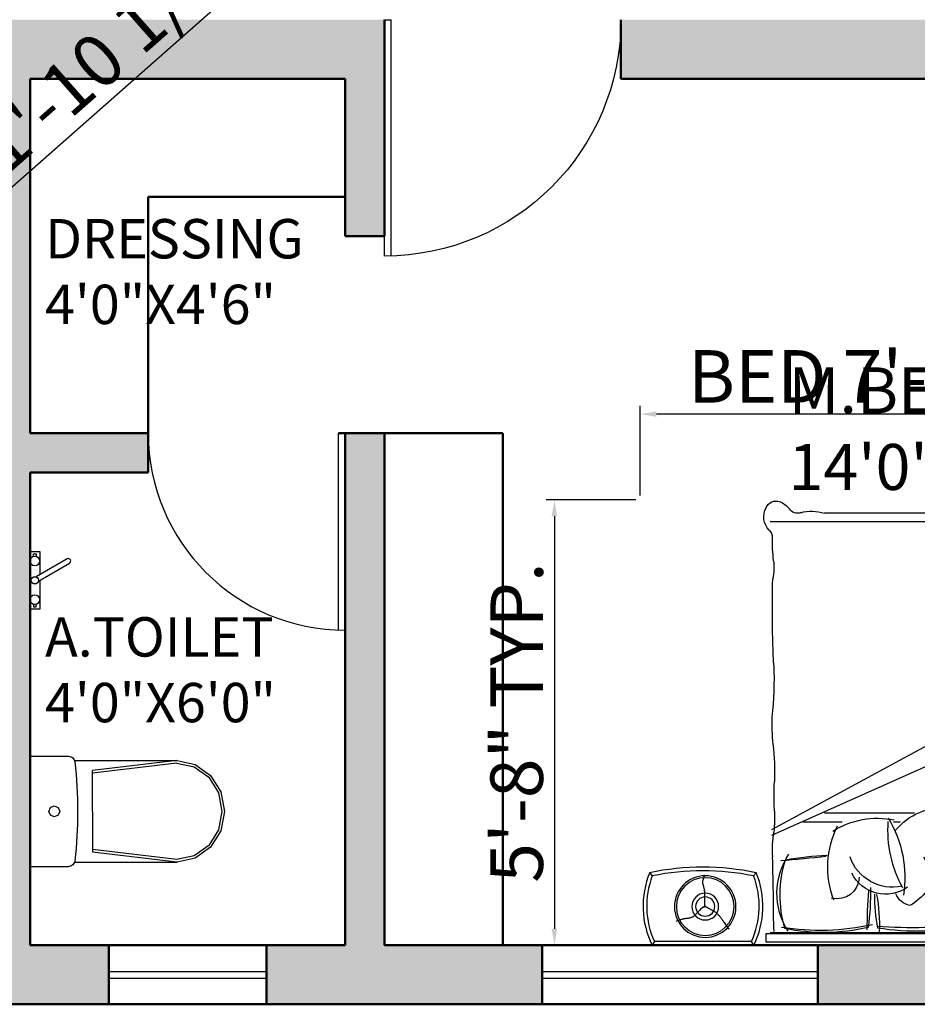
# Model space of a CAD drawing. Units: inches. Extents: x 3008 to 4088, y 1255 to 2137.
# Tile 23 of 30: x 3796 to 3933, y 1470 to 1620. Entities that reach past the tile are written whole.
import ezdxf

# ---------------------------------------------------------------- set-up
doc = ezdxf.new("R2010")
doc.units = ezdxf.units.IN
for name, color, linetype, lineweight in [('A-ANNO-DIMS', 2, 'Continuous', 18), ('A-AREA-IDEN', 7, 'Continuous', 18), ('A-DOOR', 4, 'Continuous', 25), ('A-FLOR-FIXT', 8, 'Continuous', 18), ('A-FURN', 8, 'Continuous', 18), ('A-GLAZ', 4, 'Continuous', 25), ('A-WALL', 7, 'Continuous', 50), ('A-WALL-PATT', 8, 'Continuous', 13)]:
    doc.layers.add(name, color=color, linetype=linetype, lineweight=lineweight)
doc.layers.add('SANTEH', color=7, linetype='Continuous')
doc.layers.add('TEFRİŞ', color=11, linetype='Continuous')
doc.styles.get("Standard").update_dxf_attribs({"font": 'arial.ttf'})
doc.dimstyles.new('ISO-25', dxfattribs={"dimtxt": 8, "dimasz": 2.5, "dimexe": 1.25, "dimexo": 0.625, "dimtad": 1, "dimdec": 1, "dimlunit": 3, "dimtxsty": 'Standard', "dimcen": 2.5, "dimadec": 0, "dimazin": 0, "dimtfac": 1, "dimtdec": 1, "dimtmove": 0, "dimatfit": 3, "dimfxl": 1, "dimarcsym": 0})

# ---------------------------------------------------------------- blocks, each defined once
blk = doc.blocks.new('D1')
for p, q in [((1805.96, 1500.36), (1805.96, 1464.36)), ((1806.96, 1500.36), (1806.96, 1464.36)), ((1805.96, 1464.36), (1806.96, 1464.36))]:
    blk.add_line(p, q)
blk.add_arc((1805.96, 1464.36), 36, 0, 90)
blk = doc.blocks.new('D2')
for p, q in [((1722.5, 1505.46), (1722.5, 1475.46)), ((1723.5, 1505.46), (1723.5, 1475.46)), ((1722.5, 1475.46), (1723.5, 1475.46))]:
    blk.add_line(p, q)
blk.add_arc((1722.5, 1475.46), 30, 0, 90)
blk = doc.blocks.new('WC 2 Symb_109')
at = {"layer": 'SANTEH'}
for p, q in [((0, 0), (0, 380)), ((0, 380), (132.4, 380)), ((153.6, 364.9), (506.8, 364.9)), ((506.3, 364.9), (215.7, 330.9)), ((506.3, 356), (215.7, 322)), ((215.7, 190), (215.7, 330.9)), ((215.7, 190), (215.7, 49.1)), ((506.3, 24), (215.7, 58)), ((506.3, 15.1), (215.7, 49.1)), ((153.8, 15.1), (506.8, 15.1)), ((0, 0), (132.4, 0))]:
    blk.add_line(p, q, dxfattribs=at)
for points in [[(154.6, 360.1), (153.9, 364.1), (152.3, 367.9), (150.2, 371.3), (147.4, 374.3), (144.1, 376.7), (140.5, 378.5), (136.5, 379.6), (132.4, 380)], [(154.6, 19.7), (158.6, 62.1), (161.4, 104.7), (163.1, 147.3), (163.7, 189.9), (163.1, 232.5), (161.4, 275.1), (158.6, 317.7), (154.6, 360.1)], [(506.3, 24), (565.5, 36.6), (615.7, 72.6), (649.2, 126.5), (661, 190), (649.2, 253.5), (615.7, 307.4), (565.5, 343.4), (506.3, 356)], [(506.8, 15.1), (569.2, 28.4), (622.2, 66.3), (657.6, 123.1), (670, 190), (657.6, 256.9), (622.2, 313.7), (569.2, 351.6), (506.8, 364.9)], [(132.4, 0), (136.5, 0.4), (140.4, 1.5), (144.1, 3.2), (147.3, 5.6), (150.1, 8.6), (152.3, 12), (153.8, 15.7), (154.6, 19.7)]]:
    blk.add_lwpolyline(points, dxfattribs=at)
blk.add_lwpolyline([(83.6, 208.5), (70.4, 203.1), (64.9, 190), (70.4, 176.9), (83.6, 171.5), (96.8, 176.9), (102.2, 190), (96.8, 203.1)], close=True, dxfattribs=at)
blk = doc.blocks.new('Faucet - kit sink top')
at = {"layer": 'SANTEH'}
for p, q in [((-5.5, -0.75), (-5.5, -1.25)), ((-4.94278, -0.75), (-5.5, -0.75)), ((-5.5, -1.25), (-4.94278, -1.25)), ((-0.14775, -1.7441), (3.56698, -8.1782)), ((4.43301, -7.6782), (0.71828, -1.2441)), ((4.94278, -0.75), (5.5, -0.75)), ((5.5, -1.25), (4.94278, -1.25)), ((5.5, -0.75), (5.5, -1.25))]:
    blk.add_line(p, q, dxfattribs=at)
blk.add_lwpolyline([(-0.00587, -2), (-6, -2), (-6, 0), (6, 0), (6, -2), (1.15195, -2)], dxfattribs=at)
for centre, radius in [((-4, -1), 1), ((4, -1), 1), ((0, -1), 0.75)]:
    blk.add_circle(centre, radius, dxfattribs=at)
blk.add_arc((4, -7.9282), 0.5, 210, 30, dxfattribs=at)
blk = doc.blocks.new('BED')
at = {"layer": 'TEFRİŞ'}
for p, q in [((2114.88, 1835.66), (2129.12, 1835.66)), ((2130.81, 1834.34), (2130.81, 1835.55)), ((2130.91, 1835.55), (2175.56, 1835.55)), ((2175.56, 1835.55), (2175.56, 1834.34)), ((2177.29, 1835.98), (2177.61, 1835.47)), ((2177.29, 1835.98), (2191.52, 1835.98)), ((2191.2, 1835.47), (2191.52, 1835.98)), ((2115.2, 1835.15), (2128.8, 1835.15)), ((2175.56, 1834.34), (2130.81, 1834.34)), ((2175, 1834.19), (2130.91, 1834.19)), ((2177.61, 1835.47), (2191.2, 1835.47)), ((2118.49, 1833.2), (2118.34, 1833.38)), ((2118.49, 1833.2), (2118.34, 1833.38)), ((2118.63, 1833.03), (2118.49, 1833.2)), ((2118.63, 1833.03), (2118.49, 1833.2)), ((2118.75, 1832.88), (2118.63, 1833.03)), ((2118.75, 1832.88), (2118.63, 1833.03)), ((2118.86, 1832.74), (2118.75, 1832.88)), ((2118.86, 1832.74), (2118.75, 1832.88)), ((2180.9, 1833.52), (2180.75, 1833.7)), ((2180.9, 1833.52), (2180.75, 1833.7)), ((2181.04, 1833.35), (2180.9, 1833.52)), ((2181.04, 1833.35), (2180.9, 1833.52)), ((2181.16, 1833.2), (2181.04, 1833.35)), ((2181.16, 1833.2), (2181.04, 1833.35)), ((2181.26, 1833.06), (2181.16, 1833.2)), ((2181.26, 1833.06), (2181.16, 1833.2)), ((2181.36, 1832.93), (2181.26, 1833.06)), ((2181.36, 1832.93), (2181.26, 1833.06)), ((2181.44, 1832.8), (2181.36, 1832.93)), ((2181.44, 1832.8), (2181.36, 1832.93)), ((2181.52, 1832.69), (2181.44, 1832.8)), ((2181.52, 1832.69), (2181.44, 1832.8)), ((2118.95, 1832.61), (2118.86, 1832.74)), ((2118.95, 1832.61), (2118.86, 1832.74)), ((2119.04, 1832.48), (2118.95, 1832.61)), ((2119.04, 1832.48), (2118.95, 1832.61)), ((2119.12, 1832.37), (2119.04, 1832.48)), ((2119.12, 1832.37), (2119.04, 1832.48)), ((2119.19, 1832.26), (2119.12, 1832.37)), ((2119.19, 1832.26), (2119.12, 1832.37)), ((2119.26, 1832.16), (2119.19, 1832.26)), ((2119.26, 1832.16), (2119.19, 1832.26)), ((2119.32, 1832.06), (2119.26, 1832.16)), ((2119.32, 1832.06), (2119.26, 1832.16)), ((2119.39, 1831.97), (2119.32, 1832.06)), ((2119.39, 1831.97), (2119.32, 1832.06)), ((2119.45, 1831.89), (2119.39, 1831.97)), ((2119.45, 1831.89), (2119.39, 1831.97)), ((2119.51, 1831.81), (2119.45, 1831.89)), ((2119.51, 1831.81), (2119.45, 1831.89)), ((2119.57, 1831.73), (2119.51, 1831.81)), ((2119.57, 1831.73), (2119.51, 1831.81)), ((2119.63, 1831.65), (2119.57, 1831.73)), ((2119.63, 1831.65), (2119.57, 1831.73)), ((2119.69, 1831.58), (2119.63, 1831.65)), ((2119.69, 1831.58), (2119.63, 1831.65)), ((2119.75, 1831.51), (2119.69, 1831.58)), ((2119.75, 1831.51), (2119.69, 1831.58)), ((2119.81, 1831.44), (2119.75, 1831.51)), ((2119.81, 1831.44), (2119.75, 1831.51)), ((2119.87, 1831.38), (2119.81, 1831.44)), ((2119.87, 1831.38), (2119.81, 1831.44)), ((2123.01, 1831.33), (2123.08, 1831.4)), ((2123.01, 1831.33), (2123.08, 1831.4)), ((2123.08, 1831.4), (2123.14, 1831.46)), ((2123.08, 1831.4), (2123.14, 1831.46)), ((2123.14, 1831.46), (2123.21, 1831.52)), ((2123.14, 1831.46), (2123.21, 1831.52)), ((2123.21, 1831.52), (2123.27, 1831.58)), ((2123.21, 1831.52), (2123.27, 1831.58)), ((2123.27, 1831.58), (2123.34, 1831.63)), ((2123.27, 1831.58), (2123.34, 1831.63)), ((2123.34, 1831.63), (2123.41, 1831.67)), ((2123.34, 1831.63), (2123.41, 1831.67)), ((2123.41, 1831.67), (2123.48, 1831.71)), ((2123.41, 1831.67), (2123.48, 1831.71)), ((2123.48, 1831.71), (2123.55, 1831.74)), ((2123.48, 1831.71), (2123.55, 1831.74)), ((2123.55, 1831.74), (2123.62, 1831.77)), ((2123.55, 1831.74), (2123.62, 1831.77)), ((2123.62, 1831.77), (2123.69, 1831.8)), ((2123.62, 1831.77), (2123.69, 1831.8)), ((2123.69, 1831.8), (2123.77, 1831.82)), ((2123.69, 1831.8), (2123.77, 1831.82)), ((2123.77, 1831.82), (2123.84, 1831.84)), ((2123.77, 1831.82), (2123.84, 1831.84)), ((2123.84, 1831.84), (2123.91, 1831.86)), ((2123.84, 1831.84), (2123.91, 1831.86)), ((2123.91, 1831.86), (2123.98, 1831.87)), ((2123.91, 1831.86), (2123.98, 1831.87)), ((2123.98, 1831.87), (2124.06, 1831.89)), ((2123.98, 1831.87), (2124.06, 1831.89)), ((2124.06, 1831.89), (2124.13, 1831.9)), ((2124.06, 1831.89), (2124.13, 1831.9)), ((2124.13, 1831.9), (2124.2, 1831.91)), ((2124.13, 1831.9), (2124.2, 1831.91)), ((2124.2, 1831.91), (2124.27, 1831.91)), ((2124.2, 1831.91), (2124.27, 1831.91)), ((2124.27, 1831.91), (2124.35, 1831.92)), ((2124.27, 1831.91), (2124.35, 1831.92)), ((2124.35, 1831.92), (2124.42, 1831.93)), ((2124.35, 1831.92), (2124.42, 1831.93)), ((2124.42, 1831.93), (2124.49, 1831.94)), ((2124.42, 1831.93), (2124.49, 1831.94)), ((2124.49, 1831.94), (2124.56, 1831.95)), ((2124.49, 1831.94), (2124.56, 1831.95)), ((2124.56, 1831.95), (2124.64, 1831.96)), ((2124.56, 1831.95), (2124.64, 1831.96)), ((2124.64, 1831.96), (2124.71, 1831.98)), ((2124.64, 1831.96), (2124.71, 1831.98)), ((2124.71, 1831.98), (2124.79, 1831.99)), ((2124.71, 1831.98), (2124.79, 1831.99)), ((2124.79, 1831.99), (2124.87, 1832.01)), ((2124.79, 1831.99), (2124.87, 1832.01)), ((2124.87, 1832.01), (2124.96, 1832.03)), ((2124.87, 1832.01), (2124.96, 1832.03)), ((2124.96, 1832.03), (2125.05, 1832.05)), ((2124.96, 1832.03), (2125.05, 1832.05)), ((2125.05, 1832.05), (2125.14, 1832.08)), ((2125.05, 1832.05), (2125.14, 1832.08)), ((2125.14, 1832.08), (2125.23, 1832.11)), ((2125.14, 1832.08), (2125.23, 1832.11)), ((2125.23, 1832.11), (2125.33, 1832.14)), ((2125.23, 1832.11), (2125.33, 1832.14)), ((2125.33, 1832.14), (2125.42, 1832.17)), ((2125.33, 1832.14), (2125.42, 1832.17)), ((2125.42, 1832.17), (2125.52, 1832.21)), ((2125.42, 1832.17), (2125.52, 1832.21)), ((2125.52, 1832.21), (2125.6, 1832.25)), ((2125.52, 1832.21), (2125.6, 1832.25)), ((2125.6, 1832.25), (2125.68, 1832.3)), ((2125.6, 1832.25), (2125.68, 1832.3)), ((2125.68, 1832.3), (2125.75, 1832.35)), ((2125.68, 1832.3), (2125.75, 1832.35)), ((2181.59, 1832.58), (2181.52, 1832.69)), ((2181.59, 1832.58), (2181.52, 1832.69)), ((2181.66, 1832.48), (2181.59, 1832.58)), ((2181.66, 1832.48), (2181.59, 1832.58)), ((2181.73, 1832.38), (2181.66, 1832.48)), ((2181.73, 1832.38), (2181.66, 1832.48)), ((2181.79, 1832.29), (2181.73, 1832.38)), ((2181.79, 1832.29), (2181.73, 1832.38)), ((2181.85, 1832.21), (2181.79, 1832.29)), ((2181.85, 1832.21), (2181.79, 1832.29)), ((2181.92, 1832.13), (2181.85, 1832.21)), ((2181.92, 1832.13), (2181.85, 1832.21)), ((2181.97, 1832.05), (2181.92, 1832.13)), ((2181.97, 1832.05), (2181.92, 1832.13)), ((2182.03, 1831.97), (2181.97, 1832.05)), ((2182.03, 1831.97), (2181.97, 1832.05)), ((2182.09, 1831.9), (2182.03, 1831.97)), ((2182.09, 1831.9), (2182.03, 1831.97)), ((2182.15, 1831.83), (2182.09, 1831.9)), ((2182.15, 1831.83), (2182.09, 1831.9)), ((2182.21, 1831.76), (2182.15, 1831.83)), ((2182.21, 1831.76), (2182.15, 1831.83)), ((2182.27, 1831.7), (2182.21, 1831.76)), ((2182.27, 1831.7), (2182.21, 1831.76)), ((2182.33, 1831.63), (2182.27, 1831.7)), ((2182.33, 1831.63), (2182.27, 1831.7)), ((2182.4, 1831.57), (2182.33, 1831.63)), ((2182.4, 1831.57), (2182.33, 1831.63)), ((2182.46, 1831.52), (2182.4, 1831.57)), ((2182.46, 1831.52), (2182.4, 1831.57)), ((2182.52, 1831.46), (2182.46, 1831.52)), ((2182.52, 1831.46), (2182.46, 1831.52)), ((2182.59, 1831.41), (2182.52, 1831.46)), ((2182.59, 1831.41), (2182.52, 1831.46)), ((2182.66, 1831.36), (2182.59, 1831.41)), ((2182.66, 1831.36), (2182.59, 1831.41)), ((2185.13, 1831.33), (2185.21, 1831.41)), ((2185.13, 1831.33), (2185.21, 1831.41)), ((2185.21, 1831.41), (2185.28, 1831.5)), ((2185.21, 1831.41), (2185.28, 1831.5)), ((2185.28, 1831.5), (2185.35, 1831.58)), ((2185.28, 1831.5), (2185.35, 1831.58)), ((2185.35, 1831.58), (2185.42, 1831.65)), ((2185.35, 1831.58), (2185.42, 1831.65)), ((2185.42, 1831.65), (2185.48, 1831.72)), ((2185.42, 1831.65), (2185.48, 1831.72)), ((2185.48, 1831.72), (2185.55, 1831.78)), ((2185.48, 1831.72), (2185.55, 1831.78)), ((2185.55, 1831.78), (2185.61, 1831.84)), ((2185.55, 1831.78), (2185.61, 1831.84)), ((2185.61, 1831.84), (2185.68, 1831.9)), ((2185.61, 1831.84), (2185.68, 1831.9)), ((2185.68, 1831.9), (2185.75, 1831.95)), ((2185.68, 1831.9), (2185.75, 1831.95)), ((2185.75, 1831.95), (2185.82, 1831.99)), ((2185.75, 1831.95), (2185.82, 1831.99)), ((2185.82, 1831.99), (2185.89, 1832.03)), ((2185.82, 1831.99), (2185.89, 1832.03)), ((2185.89, 1832.03), (2185.96, 1832.06)), ((2185.89, 1832.03), (2185.96, 1832.06)), ((2185.96, 1832.06), (2186.03, 1832.09)), ((2185.96, 1832.06), (2186.03, 1832.09)), ((2186.03, 1832.09), (2186.1, 1832.12)), ((2186.03, 1832.09), (2186.1, 1832.12)), ((2186.1, 1832.12), (2186.17, 1832.14)), ((2186.1, 1832.12), (2186.17, 1832.14)), ((2186.17, 1832.14), (2186.24, 1832.16)), ((2186.17, 1832.14), (2186.24, 1832.16)), ((2186.24, 1832.16), (2186.32, 1832.18)), ((2186.24, 1832.16), (2186.32, 1832.18)), ((2186.32, 1832.18), (2186.39, 1832.19)), ((2186.32, 1832.18), (2186.39, 1832.19)), ((2186.39, 1832.19), (2186.46, 1832.21)), ((2186.39, 1832.19), (2186.46, 1832.21)), ((2186.46, 1832.21), (2186.53, 1832.22)), ((2186.46, 1832.21), (2186.53, 1832.22)), ((2186.53, 1832.22), (2186.61, 1832.23)), ((2186.53, 1832.22), (2186.61, 1832.23)), ((2186.61, 1832.23), (2186.68, 1832.23)), ((2186.61, 1832.23), (2186.68, 1832.23)), ((2186.68, 1832.23), (2186.75, 1832.24)), ((2186.68, 1832.23), (2186.75, 1832.24)), ((2186.75, 1832.24), (2186.82, 1832.25)), ((2186.75, 1832.24), (2186.82, 1832.25)), ((2186.82, 1832.25), (2186.9, 1832.26)), ((2186.82, 1832.25), (2186.9, 1832.26)), ((2186.9, 1832.26), (2186.97, 1832.27)), ((2186.9, 1832.26), (2186.97, 1832.27)), ((2186.97, 1832.27), (2187.04, 1832.28)), ((2186.97, 1832.27), (2187.04, 1832.28)), ((2187.04, 1832.28), (2187.12, 1832.3)), ((2187.04, 1832.28), (2187.12, 1832.3)), ((2187.12, 1832.3), (2187.2, 1832.31)), ((2187.12, 1832.3), (2187.2, 1832.31)), ((2187.2, 1832.31), (2187.28, 1832.33)), ((2187.2, 1832.31), (2187.28, 1832.33)), ((2187.28, 1832.33), (2187.36, 1832.35)), ((2187.28, 1832.33), (2187.36, 1832.35)), ((2187.36, 1832.35), (2187.45, 1832.37)), ((2187.36, 1832.35), (2187.45, 1832.37)), ((2187.45, 1832.37), (2187.54, 1832.4)), ((2187.45, 1832.37), (2187.54, 1832.4)), ((2187.54, 1832.4), (2187.64, 1832.43)), ((2187.54, 1832.4), (2187.64, 1832.43)), ((2187.64, 1832.43), (2187.74, 1832.46)), ((2187.64, 1832.43), (2187.74, 1832.46)), ((2187.74, 1832.46), (2187.83, 1832.49)), ((2187.74, 1832.46), (2187.83, 1832.49)), ((2187.83, 1832.49), (2187.92, 1832.53)), ((2187.83, 1832.49), (2187.92, 1832.53)), ((2187.92, 1832.53), (2188.01, 1832.57)), ((2187.92, 1832.53), (2188.01, 1832.57)), ((2188.01, 1832.57), (2188.09, 1832.62)), ((2188.01, 1832.57), (2188.09, 1832.62)), ((2188.09, 1832.62), (2188.15, 1832.67)), ((2188.09, 1832.62), (2188.15, 1832.67)), ((2119.93, 1831.31), (2119.87, 1831.38)), ((2119.93, 1831.31), (2119.87, 1831.38)), ((2119.99, 1831.25), (2119.93, 1831.31)), ((2119.99, 1831.25), (2119.93, 1831.31)), ((2120.05, 1831.2), (2119.99, 1831.25)), ((2120.05, 1831.2), (2119.99, 1831.25)), ((2120.12, 1831.14), (2120.05, 1831.2)), ((2120.12, 1831.14), (2120.05, 1831.2)), ((2120.18, 1831.09), (2120.12, 1831.14)), ((2120.18, 1831.09), (2120.12, 1831.14)), ((2120.25, 1831.04), (2120.18, 1831.09)), ((2120.25, 1831.04), (2120.18, 1831.09)), ((2120.32, 1830.99), (2120.25, 1831.04)), ((2120.32, 1830.99), (2120.25, 1831.04)), ((2120.39, 1830.94), (2120.32, 1830.99)), ((2120.39, 1830.94), (2120.32, 1830.99)), ((2120.47, 1830.9), (2120.39, 1830.94)), ((2120.47, 1830.9), (2120.39, 1830.94)), ((2120.54, 1830.85), (2120.47, 1830.9)), ((2120.54, 1830.85), (2120.47, 1830.9)), ((2120.62, 1830.8), (2120.54, 1830.85)), ((2120.62, 1830.8), (2120.54, 1830.85)), ((2120.7, 1830.75), (2120.62, 1830.8)), ((2120.7, 1830.75), (2120.62, 1830.8)), ((2120.79, 1830.7), (2120.7, 1830.75)), ((2120.79, 1830.7), (2120.7, 1830.75)), ((2120.88, 1830.65), (2120.79, 1830.7)), ((2120.88, 1830.65), (2120.79, 1830.7)), ((2120.98, 1830.59), (2120.88, 1830.65)), ((2120.98, 1830.59), (2120.88, 1830.65)), ((2121.09, 1830.52), (2120.98, 1830.59)), ((2121.09, 1830.52), (2120.98, 1830.59)), ((2121.21, 1830.45), (2121.09, 1830.52)), ((2121.21, 1830.45), (2121.09, 1830.52)), ((2121.34, 1830.38), (2121.21, 1830.45)), ((2121.34, 1830.38), (2121.21, 1830.45)), ((2121.49, 1830.29), (2121.34, 1830.38)), ((2121.49, 1830.29), (2121.34, 1830.38)), ((2121.66, 1830.21), (2121.49, 1830.29)), ((2121.66, 1830.21), (2121.49, 1830.29)), ((2121.66, 1830.18), (2121.87, 1830.29)), ((2121.66, 1830.18), (2121.87, 1830.29)), ((2121.85, 1830.11), (2121.66, 1830.21)), ((2121.85, 1830.11), (2121.66, 1830.21)), ((2121.76, 1830.38), (2121.74, 1830.17)), ((2121.76, 1830.38), (2121.74, 1830.17)), ((2121.74, 1830.17), (2121.74, 1829.99)), ((2121.74, 1830.17), (2121.74, 1829.99)), ((2121.87, 1830.29), (2122.04, 1830.4)), ((2121.87, 1830.29), (2122.04, 1830.4)), ((2122.04, 1830.4), (2122.2, 1830.51)), ((2122.04, 1830.4), (2122.2, 1830.51)), ((2122.2, 1830.51), (2122.33, 1830.61)), ((2122.2, 1830.51), (2122.33, 1830.61)), ((2122.33, 1830.61), (2122.45, 1830.72)), ((2122.33, 1830.61), (2122.45, 1830.72)), ((2122.45, 1830.72), (2122.55, 1830.82)), ((2122.45, 1830.72), (2122.55, 1830.82)), ((2122.55, 1830.82), (2122.64, 1830.91)), ((2122.55, 1830.82), (2122.64, 1830.91)), ((2122.64, 1830.91), (2122.72, 1831.01)), ((2122.64, 1830.91), (2122.72, 1831.01)), ((2122.72, 1831.01), (2122.8, 1831.09)), ((2122.72, 1831.01), (2122.8, 1831.09)), ((2122.8, 1831.09), (2122.87, 1831.18)), ((2122.8, 1831.09), (2122.87, 1831.18)), ((2122.87, 1831.18), (2122.94, 1831.26)), ((2122.87, 1831.18), (2122.94, 1831.26)), ((2122.94, 1831.26), (2123.01, 1831.33)), ((2122.94, 1831.26), (2123.01, 1831.33)), ((2182.73, 1831.31), (2182.66, 1831.36)), ((2182.73, 1831.31), (2182.66, 1831.36)), ((2182.8, 1831.26), (2182.73, 1831.31)), ((2182.8, 1831.26), (2182.73, 1831.31)), ((2182.87, 1831.22), (2182.8, 1831.26)), ((2182.87, 1831.22), (2182.8, 1831.26)), ((2182.95, 1831.17), (2182.87, 1831.22)), ((2182.95, 1831.17), (2182.87, 1831.22)), ((2183.03, 1831.12), (2182.95, 1831.17)), ((2183.03, 1831.12), (2182.95, 1831.17)), ((2183.11, 1831.07), (2183.03, 1831.12)), ((2183.11, 1831.07), (2183.03, 1831.12)), ((2183.2, 1831.02), (2183.11, 1831.07)), ((2183.2, 1831.02), (2183.11, 1831.07)), ((2183.29, 1830.97), (2183.2, 1831.02)), ((2183.29, 1830.97), (2183.2, 1831.02)), ((2183.39, 1830.91), (2183.29, 1830.97)), ((2183.39, 1830.91), (2183.29, 1830.97)), ((2183.49, 1830.84), (2183.39, 1830.91)), ((2183.49, 1830.84), (2183.39, 1830.91)), ((2183.61, 1830.77), (2183.49, 1830.84)), ((2183.61, 1830.77), (2183.49, 1830.84)), ((2183.75, 1830.7), (2183.61, 1830.77)), ((2183.75, 1830.7), (2183.61, 1830.77)), ((2183.9, 1830.61), (2183.75, 1830.7)), ((2183.9, 1830.61), (2183.75, 1830.7)), ((2184.06, 1830.53), (2183.9, 1830.61)), ((2184.06, 1830.53), (2183.9, 1830.61)), ((2184.25, 1830.43), (2184.06, 1830.53)), ((2184.25, 1830.43), (2184.06, 1830.53)), ((2184.07, 1830.5), (2184.27, 1830.61)), ((2184.07, 1830.5), (2184.27, 1830.61)), ((2184.15, 1830.49), (2184.14, 1830.31)), ((2184.15, 1830.49), (2184.14, 1830.31)), ((2184.14, 1830.31), (2184.14, 1830.15)), ((2184.14, 1830.31), (2184.14, 1830.15)), ((2184.14, 1830.15), (2184.14, 1830.01)), ((2184.14, 1830.15), (2184.14, 1830.01)), ((2184.17, 1830.7), (2184.15, 1830.49)), ((2184.17, 1830.7), (2184.15, 1830.49)), ((2184.27, 1830.61), (2184.45, 1830.72)), ((2184.27, 1830.61), (2184.45, 1830.72)), ((2184.45, 1830.72), (2184.6, 1830.83)), ((2184.45, 1830.72), (2184.6, 1830.83)), ((2184.6, 1830.83), (2184.74, 1830.93)), ((2184.6, 1830.83), (2184.74, 1830.93)), ((2184.74, 1830.93), (2184.85, 1831.04)), ((2184.74, 1830.93), (2184.85, 1831.04)), ((2184.85, 1831.04), (2184.95, 1831.14)), ((2184.85, 1831.04), (2184.95, 1831.14)), ((2184.95, 1831.14), (2185.05, 1831.23)), ((2184.95, 1831.14), (2185.05, 1831.23)), ((2185.05, 1831.23), (2185.13, 1831.33)), ((2185.05, 1831.23), (2185.13, 1831.33)), ((2121.74, 1829.99), (2121.73, 1829.83)), ((2121.74, 1829.99), (2121.73, 1829.83)), ((2121.73, 1829.83), (2121.73, 1829.69)), ((2121.73, 1829.83), (2121.73, 1829.69)), ((2121.73, 1829.69), (2121.73, 1829.57)), ((2121.73, 1829.69), (2121.73, 1829.57)), ((2121.73, 1829.57), (2121.73, 1829.45)), ((2121.73, 1829.57), (2121.73, 1829.45)), ((2121.73, 1829.45), (2121.74, 1829.35)), ((2121.73, 1829.45), (2121.74, 1829.35)), ((2121.74, 1828.89), (2121.73, 1828.8)), ((2121.74, 1828.89), (2121.73, 1828.8)), ((2121.73, 1828.8), (2121.73, 1828.72)), ((2121.73, 1828.8), (2121.73, 1828.72)), ((2121.73, 1828.72), (2121.73, 1828.64)), ((2121.73, 1828.72), (2121.73, 1828.64)), ((2121.73, 1828.64), (2121.73, 1828.56)), ((2121.73, 1828.64), (2121.73, 1828.56)), ((2121.74, 1829.35), (2121.74, 1829.25)), ((2121.74, 1829.35), (2121.74, 1829.25)), ((2121.74, 1829.25), (2121.74, 1829.16)), ((2121.74, 1829.25), (2121.74, 1829.16)), ((2121.74, 1829.16), (2121.74, 1829.06)), ((2121.74, 1829.16), (2121.74, 1829.06)), ((2121.74, 1829.06), (2121.74, 1828.97)), ((2121.74, 1829.06), (2121.74, 1828.97)), ((2121.74, 1828.97), (2121.74, 1828.89)), ((2121.74, 1828.97), (2121.74, 1828.89)), ((2184.14, 1829.04), (2184.13, 1828.96)), ((2184.14, 1829.04), (2184.13, 1828.96)), ((2184.13, 1828.96), (2184.13, 1828.88)), ((2184.13, 1828.96), (2184.13, 1828.88)), ((2184.13, 1828.88), (2184.13, 1828.8)), ((2184.13, 1828.88), (2184.13, 1828.8)), ((2184.13, 1828.8), (2184.14, 1828.72)), ((2184.13, 1828.8), (2184.14, 1828.72)), ((2184.14, 1830.01), (2184.14, 1829.89)), ((2184.14, 1830.01), (2184.14, 1829.89)), ((2184.14, 1829.89), (2184.14, 1829.77)), ((2184.14, 1829.89), (2184.14, 1829.77)), ((2184.14, 1829.77), (2184.14, 1829.67)), ((2184.14, 1829.77), (2184.14, 1829.67)), ((2184.14, 1829.67), (2184.15, 1829.57)), ((2184.14, 1829.67), (2184.15, 1829.57)), ((2184.15, 1829.38), (2184.14, 1829.29)), ((2184.15, 1829.38), (2184.14, 1829.29)), ((2184.14, 1829.29), (2184.14, 1829.21)), ((2184.14, 1829.29), (2184.14, 1829.21)), ((2184.14, 1829.21), (2184.14, 1829.12)), ((2184.14, 1829.21), (2184.14, 1829.12)), ((2184.14, 1829.12), (2184.14, 1829.04)), ((2184.14, 1829.12), (2184.14, 1829.04)), ((2184.14, 1828.72), (2184.14, 1828.65)), ((2184.14, 1828.72), (2184.14, 1828.65)), ((2184.14, 1828.65), (2184.15, 1828.57)), ((2184.14, 1828.65), (2184.15, 1828.57)), ((2184.15, 1829.57), (2184.15, 1829.48)), ((2184.15, 1829.57), (2184.15, 1829.48)), ((2184.15, 1829.48), (2184.15, 1829.38)), ((2184.15, 1829.48), (2184.15, 1829.38)), ((2121.73, 1828.56), (2121.73, 1828.48)), ((2121.73, 1828.56), (2121.73, 1828.48)), ((2121.73, 1828.48), (2121.73, 1828.4)), ((2121.73, 1828.48), (2121.73, 1828.4)), ((2121.73, 1828.4), (2121.73, 1828.33)), ((2121.73, 1828.4), (2121.73, 1828.33)), ((2121.73, 1828.33), (2121.74, 1828.25)), ((2121.73, 1828.33), (2121.74, 1828.25)), ((2121.74, 1828.25), (2121.75, 1828.18)), ((2121.74, 1828.25), (2121.75, 1828.18)), ((2121.75, 1828.18), (2121.75, 1828.1)), ((2121.75, 1828.18), (2121.75, 1828.1)), ((2121.75, 1828.1), (2121.76, 1828.03)), ((2121.75, 1828.1), (2121.76, 1828.03)), ((2121.76, 1828.03), (2121.78, 1827.95)), ((2121.76, 1828.03), (2121.78, 1827.95)), ((2121.78, 1827.95), (2121.79, 1827.88)), ((2121.78, 1827.95), (2121.79, 1827.88)), ((2121.79, 1827.88), (2121.8, 1827.8)), ((2121.79, 1827.88), (2121.8, 1827.8)), ((2121.8, 1827.8), (2121.82, 1827.72)), ((2121.8, 1827.8), (2121.82, 1827.72)), ((2121.82, 1827.72), (2121.84, 1827.65)), ((2121.82, 1827.72), (2121.84, 1827.65)), ((2121.84, 1827.65), (2121.85, 1827.57)), ((2121.84, 1827.65), (2121.85, 1827.57)), ((2121.85, 1827.57), (2121.87, 1827.49)), ((2121.85, 1827.57), (2121.87, 1827.49)), ((2121.87, 1827.49), (2121.89, 1827.41)), ((2121.87, 1827.49), (2121.89, 1827.41)), ((2121.89, 1827.41), (2121.91, 1827.33)), ((2121.89, 1827.41), (2121.91, 1827.33)), ((2121.91, 1827.33), (2121.93, 1827.26)), ((2121.91, 1827.33), (2121.93, 1827.26)), ((2184.15, 1828.57), (2184.15, 1828.5)), ((2184.15, 1828.57), (2184.15, 1828.5)), ((2184.15, 1828.5), (2184.16, 1828.42)), ((2184.15, 1828.5), (2184.16, 1828.42)), ((2184.16, 1828.42), (2184.17, 1828.35)), ((2184.16, 1828.42), (2184.17, 1828.35)), ((2184.17, 1828.35), (2184.18, 1828.27)), ((2184.17, 1828.35), (2184.18, 1828.27)), ((2184.18, 1828.27), (2184.19, 1828.2)), ((2184.18, 1828.27), (2184.19, 1828.2)), ((2184.19, 1828.2), (2184.21, 1828.12)), ((2184.19, 1828.2), (2184.21, 1828.12)), ((2184.21, 1828.12), (2184.22, 1828.04)), ((2184.21, 1828.12), (2184.22, 1828.04)), ((2184.22, 1828.04), (2184.24, 1827.97)), ((2184.22, 1828.04), (2184.24, 1827.97)), ((2184.24, 1827.97), (2184.26, 1827.89)), ((2184.24, 1827.97), (2184.26, 1827.89)), ((2184.26, 1827.89), (2184.28, 1827.81)), ((2184.26, 1827.89), (2184.28, 1827.81)), ((2184.28, 1827.81), (2184.3, 1827.73)), ((2184.28, 1827.81), (2184.3, 1827.73)), ((2184.3, 1827.73), (2184.32, 1827.65)), ((2184.3, 1827.73), (2184.32, 1827.65)), ((2184.32, 1827.65), (2184.34, 1827.58)), ((2184.32, 1827.65), (2184.34, 1827.58)), ((2184.34, 1827.58), (2184.36, 1827.5)), ((2184.34, 1827.58), (2184.36, 1827.5)), ((2184.36, 1827.5), (2184.38, 1827.41)), ((2184.36, 1827.5), (2184.38, 1827.41)), ((2184.38, 1827.41), (2184.4, 1827.33)), ((2184.38, 1827.41), (2184.4, 1827.33)), ((2184.4, 1827.33), (2184.41, 1827.25)), ((2184.4, 1827.33), (2184.41, 1827.25)), ((2121.78, 1825.93), (2121.74, 1825.8)), ((2121.78, 1825.93), (2121.74, 1825.8)), ((2121.83, 1826.06), (2121.78, 1825.93)), ((2121.83, 1826.06), (2121.78, 1825.93)), ((2121.87, 1826.19), (2121.83, 1826.06)), ((2121.87, 1826.19), (2121.83, 1826.06)), ((2121.91, 1826.31), (2121.87, 1826.19)), ((2121.91, 1826.31), (2121.87, 1826.19)), ((2121.95, 1826.42), (2121.91, 1826.31)), ((2121.95, 1826.42), (2121.91, 1826.31)), ((2121.93, 1827.26), (2121.95, 1827.18)), ((2121.93, 1827.26), (2121.95, 1827.18)), ((2121.95, 1827.18), (2121.97, 1827.09)), ((2121.95, 1827.18), (2121.97, 1827.09)), ((2121.97, 1826.54), (2121.95, 1826.42)), ((2121.97, 1826.54), (2121.95, 1826.42)), ((2121.97, 1827.09), (2121.99, 1827.01)), ((2121.97, 1827.09), (2121.99, 1827.01)), ((2121.99, 1826.64), (2121.97, 1826.54)), ((2121.99, 1826.64), (2121.97, 1826.54)), ((2121.99, 1827.01), (2122, 1826.93)), ((2121.99, 1827.01), (2122, 1826.93)), ((2122, 1826.74), (2121.99, 1826.64)), ((2122, 1826.74), (2121.99, 1826.64)), ((2122, 1826.93), (2122.01, 1826.84)), ((2122, 1826.93), (2122.01, 1826.84)), ((2122.01, 1826.84), (2122, 1826.74)), ((2122.01, 1826.84), (2122, 1826.74)), ((2129.46, 1825.49), (2129.09, 1825.93)), ((2176.94, 1825.81), (2177.31, 1826.25)), ((2184.19, 1826.25), (2184.14, 1826.12)), ((2184.19, 1826.25), (2184.14, 1826.12)), ((2184.23, 1826.38), (2184.19, 1826.25)), ((2184.23, 1826.38), (2184.19, 1826.25)), ((2184.28, 1826.51), (2184.23, 1826.38)), ((2184.28, 1826.51), (2184.23, 1826.38)), ((2184.32, 1826.63), (2184.28, 1826.51)), ((2184.32, 1826.63), (2184.28, 1826.51)), ((2184.35, 1826.74), (2184.32, 1826.63)), ((2184.35, 1826.74), (2184.32, 1826.63)), ((2184.38, 1826.86), (2184.35, 1826.74)), ((2184.38, 1826.86), (2184.35, 1826.74)), ((2184.4, 1826.96), (2184.38, 1826.86)), ((2184.4, 1826.96), (2184.38, 1826.86)), ((2184.41, 1827.06), (2184.4, 1826.96)), ((2184.41, 1827.06), (2184.4, 1826.96)), ((2184.41, 1827.25), (2184.41, 1827.16)), ((2184.41, 1827.25), (2184.41, 1827.16)), ((2184.41, 1827.16), (2184.41, 1827.06)), ((2184.41, 1827.16), (2184.41, 1827.06)), ((2191.87, 1825.81), (2191.5, 1826.25)), ((2174.77, 1820.53), (2130.76, 1800.91)), ((2174.77, 1819.77), (2130.6, 1795.83)), ((2140.43, 1818.69), (2131.53, 1818.69)), ((2157.71, 1818.69), (2156.77, 1818.69)), ((2170.41, 1818.69), (2164.92, 1818.69)), ((2141.43, 1817.4), (2131.53, 1817.4)), ((2149.62, 1817.4), (2145.88, 1817.4)), ((2167.36, 1817.4), (2154.77, 1817.4)), ((2175, 1776.57), (2130.11, 1776.57)), ((2138.52, 1775.41), (2167.39, 1775.41))]:
    blk.add_line(p, q, dxfattribs=at)
for centre, radius, start, end in [((2126, 1830.19), 12.39, 153.8162, 202.314), ((2118, 1830.19), 12.39, 337.686, 26.1838), ((2188.4, 1830.51), 12.39, 153.8162, 202.314), ((2180.41, 1830.51), 12.39, 337.686, 26.1838), ((2126, 1830.19), 11.88, 155.3335, 201.0157), ((2118, 1830.19), 11.88, 338.9843, 24.6665), ((2188.4, 1830.51), 11.88, 155.3335, 201.0157), ((2180.41, 1830.51), 11.88, 338.9843, 24.6665), ((2122, 1861.35), 36.12, 258.6773, 281.3227), ((2184.41, 1861.67), 36.12, 258.6773, 281.3227), ((2122, 1861.35), 36.63, 258.2443, 281.7557), ((2184.41, 1861.67), 36.63, 258.2443, 281.7557)]:
    blk.add_arc(centre, radius, start, end, dxfattribs=at)
at = {"layer": 'TEFRİŞ', "extrusion": (0, 0, -1)}
for centre, major_axis, ratio, start_param, end_param in [((2121.68, 1830.24), (-3.05, -3.05), 1, 3.926991, 10.210176), ((2121.68, 1830.24), (2.86, -2.86), 1, 5.497787, 11.780972), ((2121.68, 1830.24), (2.86, -2.86), 1, 5.497787, 11.780972), ((2206.14, 1830.73), (-52.86, -52.86), 1, 0.767743, 0.83177), ((2138.85, 1803.05), (-22.1, 22.1), 1, 0.544604, 1.006234), ((2154.12, 1796.61), (-26.46, 26.46), 1, 0.596409, 0.940188), ((2167.6, 1797.72), (-0.51, 36.47), 0.865194, -0.185965, 0.185965), ((2184.09, 1830.56), (-3.05, -3.05), 1, 3.926991, 10.210176), ((2184.09, 1830.56), (2.86, -2.86), 1, 5.497787, 11.780972), ((2184.09, 1830.56), (2.86, -2.86), 1, 5.497787, 11.780972), ((2139.43, 1773.84), (-42.35, 42.35), 1, 0.646251, 0.896949), ((2154.7, 1828.89), (-15.68, 15.68), 1, -1.00675, -0.580436), ((2181.61, 1828.44), (-34.39, 34.39), 1, -0.888486, -0.672463), ((2164.51, 1832.79), (-13.41, 13.41), 1, -0.974476, -0.730892), ((2127.6, 1828.81), (-13.23, 13.23), 1, 2.100388, 2.328052), ((2155, 1761.9), (-50.65, -50.65), 1, 2.239512, 2.426533), ((2172.01, 1828.66), (-17.93, 17.93), 1, -0.753394, -0.598744), ((2128.44, 1832.96), (-13.26, -13.26), 1, 3.889049, 4.127298), ((2183.72, 1833.22), (-17, 17), 1, -0.967105, -0.749712), ((2134, 1828.8), (-18.62, 18.62), 1, 2.173461, 2.355043), ((2168.35, 1789.27), (-1.33, 44.62), 0.875277, -0.163954, 0.163954), ((2199.2, 1828.45), (-27.06, -27.06), 1, 0.770625, 0.917228), ((2087.32, 1833.96), (-52.37, 52.37), 1, 2.358049, 2.431787), ((2164.15, 1828.7), (-6.99, 6.99), 1, 1.789136, 2.946702), ((2156.76, 1828.98), (-11.9, -11.9), 1, 3.646453, 4.226155), ((2099.77, 1830.73), (-52.86, 52.86), 1, 2.311571, 2.373849), ((2121.68, 1830.24), (1.33, -1.33), 1, 5.497787, 11.780972), ((2121.68, 1830.24), (1.33, -1.33), 1, 5.497787, 11.780972), ((2121.68, 1830.24), (0.952, -0.952), 1, 5.497787, 11.780972), ((2121.68, 1830.24), (0.952, -0.952), 1, 5.497787, 11.780972), ((2184.09, 1830.56), (1.33, -1.33), 1, 5.497787, 11.780972), ((2184.09, 1830.56), (1.33, -1.33), 1, 5.497787, 11.780972), ((2184.09, 1830.56), (0.952, -0.952), 1, 5.497787, 11.780972), ((2184.09, 1830.56), (0.952, -0.952), 1, 5.497787, 11.780972), ((2159.55, 1823.33), (-5.81, 5.81), 1, -0.516587, 0.256776), ((2154.84, 1827.75), (-1.93, 1.93), 1, 0.997904, 1.977819), ((2675.38, 1815.09), (-384.79, -384.79), 1, 0.80103, 0.811711), ((2147.44, 1824.41), (-3.36, -3.36), 1, 1.11934, 2.270556), ((2145.66, 1827.01), (-1.62, 1.62), 1, 1.310976, 2.284591), ((2172, 1826.44), (-11.23, 11.23), 1, -1.332486, -0.624868), ((2158.82, 1823.55), (-3.74, -3.74), 1, 1.730792, 3.47045), ((2166.67, 1824.96), (-2.93, 3.91), 0.760601, -0.723751, 0.723751), ((2153.88, 1825.05), (-9.22, 9.22), 1, 1.994956, 2.818753), ((1630.53, 1815.09), (-384.79, 384.79), 1, 2.329881, 2.340562), ((2140.05, 1819.86), (-5.1, 5.1), 1, 0.238357, 1.390139), ((2139.42, 1820.79), (-4.21, -4.21), 1, 1.82161, 3.349145), ((2160.6, 1825.98), (-9.68, -9.68), 1, 0.009196, 0.886853), ((2148.35, 1820.65), (-4.63, -4.63), 1, 2.117602, 3.020837), ((2141.71, 1819.83), (-11.86, 11.86), 1, 1.850844, 2.42862), ((2157.83, 1821.53), (-4.47, 4.47), 1, 0.576679, 2.021689), ((2148.15, 1825.25), (-7.14, -7.14), 1, 6.061986, 7.190757), ((2154.93, 1828.48), (-11.96, 11.96), 1, -1.530302, -0.934407), ((2147.86, 1820.64), (-4.48, 4.48), 1, 0.665914, 1.867503), ((2170.68, 1829.67), (-16.79, 16.79), 1, -1.354718, -0.902276), ((2127.37, 1815.76), (-10.68, 10.68), 1, 1.657204, 1.779381), ((2146.08, 1822.57), (-10.5, 10.5), 1, -0.951783, -0.716225), ((2132.43, 1774.09), (-35.41, -35.41), 1, 2.362911, 2.464592), ((2140.17, 1862.96), (-27.99, 27.99), 1, 3.983025, 4.107469), ((2165.73, 1860.69), (-26.41, -26.41), 1, 5.306413, 5.463767), ((2199.62, 1529.47), (-209.2, 209.2), 1, 0.675361, 0.697001), ((2159.82, 1822.57), (-10.5, -10.5), 1, 3.857817, 4.093375), ((2127.37, 1815.76), (-10.68, 10.68), 1, 1.94252, 2.248924), ((2111.06, 1818.12), (-14.48, 14.48), 1, 2.258605, 2.412359), ((2141.33, 1830.48), (-9.55, -9.55), 1, 4.941413, 5.601673), ((2150.79, 1825.18), (-6, 6), 1, 3.032122, 4.026148), ((2159.02, 1834.9), (-3.04, 16.53), 0.830169, 2.822117, 3.461068), ((2194.85, 1818.12), (-14.48, 14.48), 1, -0.841563, -0.687809), ((2169.92, 1815.01), (-27.2, -27.2), 1, 0.734393, 0.836404), ((2135.98, 1815.01), (-27.2, -27.2), 1, 3.875985, 3.977996), ((2098.24, 1811.68), (-23.54, -23.54), 1, 3.885834, 4.043401), ((2207.66, 1811.68), (-23.54, -23.54), 1, 0.668988, 0.826555), ((2189.03, 1803.74), (-40.91, -40.91), 1, 0.789771, 0.855756), ((2116.87, 1803.74), (-40.91, 40.91), 1, 2.285836, 2.351822), ((2122.14, 1803.63), (-6.39, -6.39), 1, 3.886359, 4.265474), ((2222.76, 1798.77), (-34.16, -34.16), 1, 0.743488, 0.893627), ((2135.02, 1798.41), (-3.45, 3.45), 1, -0.831635, -0.314979), ((2135.48, 1798), (-3.77, -3.77), 1, 0.329385, 0.820948), ((2127.76, 1790.23), (-1, 12.37), 0.296708, 1.141067, 2.000525), ((2148.06, 1790.38), (-0.75, 67.37), 0.394952, 1.480524, 1.661068), ((2118.49, 1784.2), (-9.24, -9.24), 1, 3.839645, 4.088086), ((2182.27, 1782.99), (-5.52, -5.52), 1, 0.671703, 0.993321), ((2162.12, 1778.86), (-21.85, 21.85), 1, -0.78611, -0.680117), ((2143.78, 1778.86), (-21.85, 21.85), 1, 2.250913, 2.356906), ((2132.72, 1775.92), (-1.91, -1.91), 1, 0.284117, 1.557111), ((2129.83, 1778.8), (-0.986, 0.986), 1, 2.330985, 3.163296), ((2176.08, 1778.8), (-0.986, 0.986), 1, 4.690686, 5.522997), ((2173.18, 1775.92), (-1.91, -1.91), 1, 3.155278, 4.428271), ((2130.83, 1777), (-2.49, -2.49), 1, 4.590984, 5.084038), ((2134.73, 1774.06), (-0.964, -0.964), 1, 1.381176, 2.701227), ((2136.75, 1781.14), (-4.24, 4.24), 1, 3.62713, 4.188813), ((2169.16, 1781.14), (-4.24, 4.24), 1, 3.665169, 4.226852), ((2171.17, 1774.06), (-0.964, -0.964), 1, 2.011162, 3.331212), ((2175.07, 1777), (-2.49, 2.49), 1, 4.34074, 4.833793), ((2131.79, 1775.28), (-1.11, 1.11), 1, 3.629269, 5.067473), ((2174.12, 1775.28), (-1.11, 1.11), 1, 2.786508, 4.224712)]:
    blk.add_ellipse(centre, major_axis=major_axis, ratio=ratio, start_param=start_param, end_param=end_param, dxfattribs=at)
blk = doc.blocks.new('*D37')
at = {"layer": 'A-ANNO-DIMS', "color": 0, "lineweight": -2, "transparency": 16777216}
for p, q in [((3890.84, 1547.21), (3890.84, 1560.88)), ((3977.82, 1547.21), (3977.82, 1560.88)), ((3975.32, 1559.63), (3893.34, 1559.63))]:
    blk.add_line(p, q, dxfattribs=at)
at = {"layer": 'A-ANNO-DIMS', "color": 0, "transparency": 16777216}
for points in [[(3893.34, 1560.04), (3893.34, 1559.21), (3890.84, 1559.63)], [(3975.32, 1560.04), (3975.32, 1559.21), (3977.82, 1559.63)]]:
    blk.add_solid(points, dxfattribs=at)
at = {"layer": 'Defpoints', "color": 0, "transparency": 16777216}
for p in [(3890.84, 1559.63), (3890.84, 1546.58), (3977.82, 1546.58)]:
    blk.add_point(p, dxfattribs=at)
at = {"layer": 'A-ANNO-DIMS', "color": 0, "transparency": 16777216, "insert": (3934.33, 1564.34), "char_height": 8, "attachment_point": 5}
blk.add_mtext('BED 7\'-3" TYP.', dxfattribs=at)
blk = doc.blocks.new('*D38')
at = {"layer": 'A-ANNO-DIMS', "color": 0, "lineweight": -2, "transparency": 16777216}
for p, q in [((3890.22, 1546.58), (3876.55, 1546.58)), ((3877.8, 1544.08), (3877.8, 1481.22)), ((3890.22, 1478.72), (3876.55, 1478.72))]:
    blk.add_line(p, q, dxfattribs=at)
at = {"layer": 'A-ANNO-DIMS', "color": 0, "transparency": 16777216}
for points in [[(3877.38, 1544.08), (3878.21, 1544.08), (3877.8, 1546.58)], [(3877.38, 1481.22), (3878.21, 1481.22), (3877.8, 1478.72)]]:
    blk.add_solid(points, dxfattribs=at)
at = {"layer": 'Defpoints', "color": 0, "transparency": 16777216}
for p in [(3890.84, 1546.58), (3877.8, 1478.72), (3890.84, 1478.72)]:
    blk.add_point(p, dxfattribs=at)
at = {"layer": 'A-ANNO-DIMS', "color": 0, "transparency": 16777216, "insert": (3873.09, 1512.65), "char_height": 8, "attachment_point": 5, "rotation": 90}
blk.add_mtext('5\'-8" TYP.', dxfattribs=at)
blk = doc.blocks.new('*D52')
at = {"layer": 'A-ANNO-DIMS', "color": 0, "lineweight": -2, "transparency": 16777216}
for p, q in [((3793.55, 1592.8), (3851.01, 1643.48)), ((3791.71, 1594.89), (3794.38, 1591.87)), ((3778.59, 1579.61), (3791.68, 1591.15)), ((3774.87, 1580.05), (3777.54, 1577.02))]:
    blk.add_line(p, q, dxfattribs=at)
at = {"layer": 'A-ANNO-DIMS', "color": 0, "transparency": 16777216}
for points in [[(3791.4, 1591.46), (3791.95, 1590.84), (3793.55, 1592.8)], [(3778.32, 1579.92), (3778.87, 1579.3), (3776.72, 1577.96)]]:
    blk.add_solid(points, dxfattribs=at)
at = {"layer": 'Defpoints', "color": 0, "transparency": 16777216}
for p in [(3791.29, 1595.36), (3793.55, 1592.8), (3774.46, 1580.52)]:
    blk.add_point(p, dxfattribs=at)
at = {"layer": 'A-ANNO-DIMS', "color": 0, "transparency": 16777216, "insert": (3820.07, 1622.54), "char_height": 8, "attachment_point": 5, "rotation": 41.4119}
blk.add_mtext('1\'-10 1/2" TYP.', dxfattribs=at)

msp = doc.modelspace()

# ---------------------------------------------------------------- hatches: boundary and pattern name
at = {"layer": 'A-WALL-PATT'}
h = msp.add_hatch(color=256, dxfattribs=at)
h.dxf.hatch_style = 1
h.paths.add_polyline_path([(3665.94, 1631.72), (3656.94, 1631.72), (3656.94, 1546.72), (3665.94, 1546.72)])
h.paths.add_polyline_path([(3851.94, 1619.72), (3701.94, 1619.72), (3701.94, 1610.72), (3788.94, 1610.72), (3788.94, 1469.72), (3809.94, 1469.72), (3809.94, 1478.72), (3797.94, 1478.72), (3797.94, 1550.72), (3815.94, 1550.72), (3815.94, 1556.72), (3797.94, 1556.72), (3797.94, 1610.72), (3845.94, 1610.72), (3845.94, 1586.72), (3851.94, 1586.72)])
h.paths.add_polyline_path([(4028.94, 1631.72), (4019.94, 1631.72), (4019.94, 1619.72), (3887.94, 1619.72), (3887.94, 1610.72), (4019.94, 1610.72), (4019.94, 1577.72), (4028.94, 1577.72)])
h.paths.add_polyline_path([(3875.94, 1478.72), (3851.94, 1478.72), (3851.94, 1556.72), (3845.94, 1556.72), (3845.94, 1526.72), (3845.94, 1478.72), (3833.94, 1478.72), (3833.94, 1469.72), (3875.94, 1469.72)])
h.paths.add_polyline_path([(3959.94, 1478.72), (3917.94, 1478.72), (3917.94, 1469.72), (3959.94, 1469.72)])
h.paths.add_polyline_path([(4028.94, 1511.72), (4019.94, 1511.72), (4019.94, 1478.72), (4001.94, 1478.72), (4001.94, 1469.72), (4028.94, 1469.72)])
h.paths.add_polyline_path([(4028.94, 1699.22), (4019.94, 1699.22), (4019.94, 1673.72), (3893.94, 1673.72), (3893.94, 1649.72), (3899.94, 1649.72), (3899.94, 1667.72), (4019.94, 1667.72), (4019.94, 1655.72), (4028.94, 1655.72)])
h.paths.add_polyline_path([(4028.94, 1847.72), (4019.94, 1847.72), (4019.94, 1796.72), (3863.94, 1796.72), (3863.94, 1790.72), (4019.94, 1790.72), (4019.94, 1765.22), (4028.94, 1765.22)])
h.paths.add_polyline_path([(3815.94, 1796.72), (3779.94, 1796.72), (3665.94, 1796.72), (3665.94, 1898.72), (3656.94, 1898.72), (3656.94, 1673.72), (3665.94, 1673.72), (3665.94, 1790.72), (3815.94, 1790.72)])
h.paths.add_polyline_path([(3755.94, 1949.72), (3656.94, 1949.72), (3656.94, 1940.72), (3665.94, 1940.72), (3755.94, 1940.72)])
h.paths.add_polyline_path([(3827.94, 1949.72), (3797.94, 1949.72), (3797.94, 1940.72), (3809.94, 1940.72), (3809.94, 1874.72), (3815.94, 1874.72), (3815.94, 1940.72), (3827.94, 1940.72)])
h.paths.add_polyline_path([(3953.94, 1949.72), (3851.94, 1949.72), (3851.94, 1940.72), (3863.94, 1940.72), (3863.94, 1844.72), (3809.94, 1844.72), (3809.94, 1832.72), (3815.94, 1832.72), (3815.94, 1838.72), (3863.94, 1838.72), (3869.94, 1838.72), (3869.94, 1940.72), (3953.94, 1940.72)])
h.paths.add_polyline_path([(4028.94, 1949.72), (3995.94, 1949.72), (3995.94, 1940.72), (4019.94, 1940.72), (4019.94, 1889.72), (4028.94, 1889.72)])

# ---------------------------------------------------------------- linework, layer by layer
at = {"layer": 'A-GLAZ'}
for p, q in [((3809.94, 1474.72), (3833.94, 1474.72)), ((3875.94, 1474.72), (3917.94, 1474.72)), ((3809.94, 1473.72), (3833.94, 1473.72)), ((3875.94, 1473.72), (3917.94, 1473.72))]:
    msp.add_line(p, q, dxfattribs=at)
at = {"layer": 'A-WALL'}
for p, q in [((3851.94, 1586.72), (3851.94, 1619.72)), ((3887.94, 1610.72), (3887.94, 1619.72)), ((3797.94, 1610.72), (3845.94, 1610.72)), ((3797.94, 1556.72), (3797.94, 1610.72)), ((3845.94, 1586.72), (3845.94, 1610.72)), ((3887.94, 1610.72), (4019.94, 1610.72)), ((3815.94, 1592.72), (3845.94, 1592.72)), ((3815.94, 1556.72), (3815.94, 1592.72)), ((3851.94, 1586.72), (3845.94, 1586.72)), ((3815.94, 1556.72), (3797.94, 1556.72)), ((3815.94, 1550.72), (3815.94, 1556.72)), ((3869.94, 1556.72), (3844.94, 1556.72)), ((3845.94, 1478.72), (3845.94, 1556.72)), ((3851.94, 1478.72), (3851.94, 1556.72)), ((3869.94, 1478.72), (3869.94, 1556.72)), ((3797.94, 1478.72), (3797.94, 1550.72)), ((3815.94, 1550.72), (3797.94, 1550.72)), ((3845.94, 1478.72), (3797.94, 1478.72)), ((3809.94, 1469.72), (3809.94, 1478.72)), ((3833.94, 1469.72), (3833.94, 1478.72)), ((4019.94, 1478.72), (3851.94, 1478.72)), ((3875.94, 1469.72), (3875.94, 1478.72)), ((3917.94, 1469.72), (3917.94, 1478.72)), ((4028.94, 1469.72), (3788.94, 1469.72))]:
    msp.add_line(p, q, dxfattribs=at)

# ---------------------------------------------------------------- block references
at = {"layer": 'A-DOOR', "xscale": -1, "rotation": 180}
msp.add_blockref('D1', (2045.98, 3084.08), dxfattribs=at)
at = {"layer": 'A-DOOR', "rotation": 180}
msp.add_blockref('D2', (5568.44, 3032.18), dxfattribs=at)
at = {"layer": 'A-FLOR-FIXT'}
for name, p, xscale, yscale, zscale, rotation in [('Faucet - kit sink top', (3797.94, 1534.31), 0.7356136897818673, 0.7356136897818673, 0.7356136897818673, 90), ('WC 2 Symb_109', (3797.94, 1507.51), -0.0441898926459964, 0.0441898926459964, 0.0441898926459964, 180)]:
    msp.add_blockref(name, p, dxfattribs=dict(at, xscale=xscale, yscale=yscale, zscale=zscale, rotation=rotation))
at = {"layer": 'A-FURN', "xscale": 1.086875874800008, "yscale": 1.086875874800008, "zscale": 1.086875874800008, "rotation": 180}
msp.add_blockref('BED', (6274.6, 3474.2), dxfattribs=at)

# ---------------------------------------------------------------- texts
at = {"layer": 'A-AREA-IDEN', "attachment_point": 1}
for s, insert, char_height in [('{\\fTimes New Roman|b0|i0|c0|p18;DRESSING\\P4\'0"X4\'6"}', (3800.23, 1589.35), 6), ('{\\fTimes New Roman|b0|i0|c0|p18;M.BEDROOM\\P14\'0"X11\'0"}', (3913.46, 1566.75), 7), ('{\\fTimes New Roman|b0|i0|c0|p18;A.TOILET\\P4\'0"X6\'0"}', (3800.23, 1528.69), 6)]:
    msp.add_mtext_dynamic_manual_height_columns(s, width=105.6127, gutter_width=12.5, heights=[0], dxfattribs=dict(at, insert=insert, char_height=char_height))

# ---------------------------------------------------------------- dimensions: what is measured, and where the dimension line sits
at = {"layer": 'A-ANNO-DIMS'}
for base, p1, p2, angle, text, picture, middle in [((3793.55, 1592.8), (3774.46, 1580.52), (3791.29, 1595.36), 41.4119, '<> TYP.', '*D52', (3820.07, 1622.54)), ((3890.84, 1559.63), (3977.82, 1546.58), (3890.84, 1546.58), 180, 'BED <> TYP.', '*D37', (3934.33, 1564.34)), ((3877.8, 1478.72), (3890.84, 1546.58), (3890.84, 1478.72), 270, '<> TYP.', '*D38', (3873.09, 1512.65))]:
    dim = msp.add_linear_dim(base=base, p1=p1, p2=p2, angle=angle, text=text, dimstyle='ISO-25', override={"dimdec": 1, "dimrnd": 0, "dimzin": 1, "dimlunit": 4, "dimfrac": 2}, dxfattribs=at)
    dim.commit()
    dim.dimension.update_dxf_attribs({"geometry": picture, "text_midpoint": middle})

doc.saveas('drawing.dxf')
